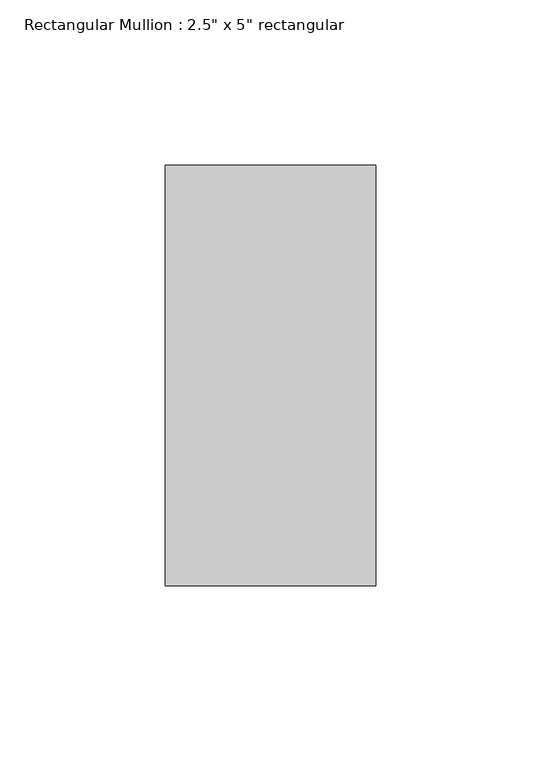
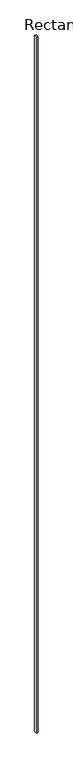
"""IFC4 building model written with IfcOpenShell, lengths in millimetres: member geometry."""

from ifc_helpers import new_model, si_unit, frame, origin, place, context, project, spatial, polyline, outline, extrude, source, transform, mapped, element, save


def member_4a4c44fd(model_context):
    return source(origin(), model_context, "Body", "SweptSolid", [
        extrude(outline(polyline([(31.75, 63.5), (31.75, -63.5), (-31.75, -63.5), (-31.75, 63.5), (31.75, 63.5)])), frame((0.0, 0.0, -29260.8), z_axis=(0.0, 0.0, 1.0), x_axis=(1.0, 0.0, 0.0)), (0.0, 0.0, 1.0), 29260.8),
    ])


if __name__ == "__main__":
    model = new_model("IFC4")
    model_context = context("Model", 3, world=origin())
    ifc_project = project(units=[si_unit("LENGTHUNIT", "METRE", prefix="MILLI")], contexts=[model_context])
    site = spatial("IfcSite", under=ifc_project)
    building = spatial("IfcBuilding", under=site)
    placement = place(None, origin())
    member_shape = member_4a4c44fd(model_context)
    element("IfcMember", 1, ObjectType="Rectangular Mullion : 2.5\" x 5\" rectangular", at=placement, inside=building, context=model_context, shape_type="MappedRepresentation", body=[
        mapped(member_shape, transform((0.0, 0.0, 0.0), x_axis=(1.0, 0.0, 0.0), y_axis=(0.0, 1.0, 0.0), z_axis=(0.0, 0.0, 1.0))),
    ])
    save(model, "model.ifc")

# Revit data of these elements
# Type "Rectangular Mullion : 2.5\" x 5\" rectangular"
#   built-in parameter 1007304 = 0.416667 (stored number, unit not read)
#   built-in parameter 1007301 = 0.104167 (stored number, unit not read)
#   built-in parameter 1007300 = 0.104167 (stored number, unit not read)
# Element 1 (IfcMember, "Rectangular Mullion : 2.5\" x 5\" rectangular")
#   Materials on its faces: "Aluminum"
# Materials
#   "Aluminum": class "Metal", colour RGB 247 247 247, transparency 0, Description = "Aluminum 6061", Cost = 0
